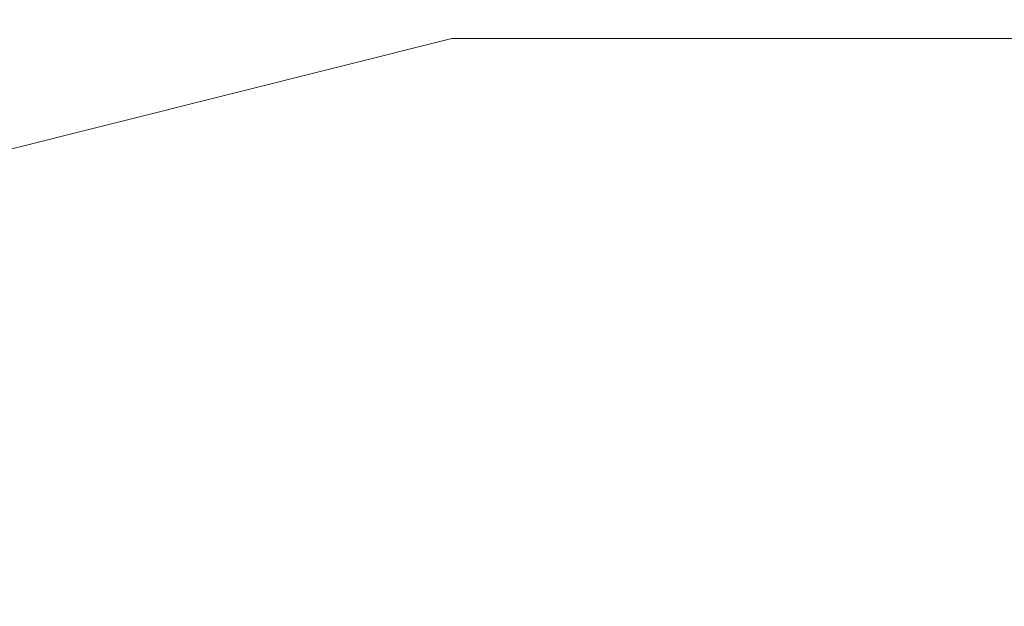
# Model space of a CAD drawing. Units: inches. Extents: x 2091 to 2899, y 967 to 2217.
# Tile 103 of 256: x 2252.951 to 2253.5204, y 1100.0709 to 1100.4099. Entities that reach past the tile are written whole.
import ezdxf

# ---------------------------------------------------------------- set-up
doc = ezdxf.new("R2010")
doc.units = ezdxf.units.IN
doc.layers.add('A-ANNO-DIMS', color=2, linetype='Continuous', lineweight=18)
doc.layers.add('L-PLNT-TREE', color=94, linetype='Continuous', lineweight=13)
doc.layers.add('A-WALL-PATT', color=141, linetype='Continuous', lineweight=13, true_color=0xadddf7)
doc.styles.get("Standard").update_dxf_attribs({"font": 'arial.ttf'})
doc.dimstyles.new('ISO-25', dxfattribs={"dimtxt": 4, "dimasz": 4, "dimexe": 1.25, "dimexo": 0.625, "dimtad": 1, "dimdec": 0, "dimlunit": 3, "dimtxsty": 'Standard', "dimcen": 2.5, "dimadec": 0, "dimazin": 0, "dimtfac": 1, "dimtdec": 0, "dimtmove": 0, "dimatfit": 3, "dimfxl": 1, "dimarcsym": 0})

# ---------------------------------------------------------------- blocks, each defined once
blk = doc.blocks.new('*U29')
for p, q in [((-402.336, 12.192), (-451.104, 0)), ((-341.376, 12.192), (-402.336, 12.192))]:
    blk.add_line(p, q)
blk = doc.blocks.new('*D71')
at = {"layer": 'A-ANNO-DIMS', "color": 0, "lineweight": -2, "transparency": 16777216}
for p, q in [((2212.1436, 1351.29406), (2212.1436, 969.4643)), ((2452.1436, 1351.29406), (2452.1436, 969.4643)), ((2216.1436, 970.7143), (2448.1436, 970.7143))]:
    blk.add_line(p, q, dxfattribs=at)
at = {"layer": 'A-ANNO-DIMS', "color": 0, "transparency": 16777216}
for points in [[(2216.1436, 971.38097), (2216.1436, 970.04764), (2212.1436, 970.7143)], [(2448.1436, 971.38097), (2448.1436, 970.04764), (2452.1436, 970.7143)]]:
    blk.add_solid(points, dxfattribs=at)
at = {"layer": 'Defpoints', "color": 0, "transparency": 16777216}
for p in [(2212.1436, 1351.91906), (2452.1436, 1351.91906), (2452.1436, 970.7143)]:
    blk.add_point(p, dxfattribs=at)
at = {"layer": 'A-ANNO-DIMS', "color": 0, "transparency": 16777216, "insert": (2332.1436, 973.38159), "char_height": 4, "attachment_point": 5}
blk.add_mtext('20\'-0"', dxfattribs=at)
blk = doc.blocks.new('*D75')
at = {"layer": 'A-ANNO-DIMS', "color": 0, "lineweight": -2, "transparency": 16777216}
for p, q in [((2212.1436, 1274.79406), (2212.1436, 969.4643)), ((2308.1436, 1274.79406), (2308.1436, 969.4643)), ((2216.1436, 970.7143), (2304.1436, 970.7143))]:
    blk.add_line(p, q, dxfattribs=at)
at = {"layer": 'A-ANNO-DIMS', "color": 0, "transparency": 16777216}
for points in [[(2216.1436, 971.38097), (2216.1436, 970.04764), (2212.1436, 970.7143)], [(2304.1436, 971.38097), (2304.1436, 970.04764), (2308.1436, 970.7143)]]:
    blk.add_solid(points, dxfattribs=at)
at = {"layer": 'Defpoints', "color": 0, "transparency": 16777216}
for p in [(2212.1436, 1275.41906), (2308.1436, 1275.41906), (2308.1436, 970.7143)]:
    blk.add_point(p, dxfattribs=at)
at = {"layer": 'A-ANNO-DIMS', "color": 0, "transparency": 16777216, "insert": (2260.1436, 973.38159), "char_height": 4, "attachment_point": 5}
blk.add_mtext('8\'-0"', dxfattribs=at)

msp = doc.modelspace()

# ---------------------------------------------------------------- hatches: boundary and pattern name
at = {"layer": 'A-WALL-PATT'}
h = msp.add_hatch(color=256, dxfattribs=at)
h.dxf.hatch_style = 1
h.paths.add_polyline_path([(2803.1436, 2050.91906), (2203.1436, 2050.91906), (2203.1436, 1090.91906), (2803.1436, 1090.91906)])
h.paths.add_polyline_path([(2635.79885, 1147.54046), (2674.52405, 1147.54046, 0.376086), (2678.52967, 1152.8802), (2678.52967, 1159.55647, 0.333335), (2674.52432, 1163.56185), (2674.52432, 1163.56185), (2674.52432, 1192.93439), (2635.80597, 1192.93439), (2597.08762, 1192.93439), (2597.08762, 1163.56185, 0.333335), (2593.08228, 1159.55647), (2593.08228, 1152.8802, 0.376086), (2597.08789, 1147.54046)], flags=0)
h.paths.add_polyline_path([(2436.01043, 1278.24078, 0.000483), (2435.95264, 1278.21503, -0.001328), (2435.93563, 1278.11169, -0.001711), (2436.11644, 1278.04076, 0.002185)], flags=0)
h.paths.add_polyline_path([(2794.1436, 1143.41906), (2794.1436, 1347.41906), (2543.37017, 1347.41906), (2543.37017, 1351.91906), (2794.1436, 1351.91906), (2794.1436, 1392.71355), (2793.9474, 1392.71355), (2793.9474, 1473.5369), (2794.1436, 1473.5369), (2794.1436, 1531.91906), (2650.1436, 1531.91906), (2650.1436, 1536.41906), (2794.1436, 1536.41906), (2794.1436, 1692.41906), (2609.37561, 1692.41906), (2609.37561, 1644.41906), (2604.87561, 1644.41906), (2604.87561, 1744.91906), (2609.37561, 1744.91906), (2609.37561, 1696.91906), (2794.1436, 1696.91906), (2794.1436, 1780.91906), (2609.6436, 1780.91906), (2493.87561, 1780.91906), (2493.87561, 1785.41906), (2609.6436, 1785.41906), (2794.1436, 1785.41906), (2794.1436, 1847.93882), (2793.95122, 1847.93882), (2793.95122, 1928.76217), (2794.1436, 1928.76217), (2794.1436, 1941.41906), (2614.1436, 1941.41906), (2614.1436, 1821.41906), (2609.6436, 1821.41906), (2609.6436, 1941.41906), (2392.1436, 1941.41906), (2392.1436, 1819.91906), (2387.6436, 1819.91906), (2387.6436, 1941.41906), (2212.1436, 1941.41906), (2212.1436, 1783.91906), (2392.1436, 1783.91906), (2392.1436, 1780.91906), (2212.1436, 1780.91906), (2212.1436, 1629.41906), (2387.6436, 1629.41906), (2387.6436, 1744.91906), (2392.1436, 1744.91906), (2392.1436, 1627.91906), (2317.1436, 1627.91906), (2317.1436, 1551.41906), (2317.1436, 1536.41906), (2459.38359, 1536.41906), (2459.38359, 1602.39648), (2463.88359, 1602.39648), (2463.88359, 1531.91906), (2456.6436, 1531.91906), (2456.6436, 1529.91906), (2452.1436, 1529.91906), (2452.1436, 1531.91906), (2312.6436, 1531.91906), (2312.6436, 1551.41906), (2306.1436, 1551.41906), (2306.1436, 1555.91906), (2308.1436, 1555.91906), (2308.1436, 1551.41906), (2312.6436, 1551.41906), (2312.6436, 1627.91906), (2212.1436, 1627.91906), (2212.1436, 1555.91906), (2270.1436, 1555.91906), (2270.1436, 1551.41906), (2212.1436, 1551.41906), (2212.1436, 1351.91906), (2272.1436, 1351.91906), (2272.1436, 1347.41906), (2212.1436, 1347.41906), (2212.1436, 1275.41906), (2308.1436, 1275.41906), (2308.1436, 1351.91906), (2452.1436, 1351.91906), (2452.1436, 1493.91906), (2456.6436, 1493.91906), (2456.6436, 1347.41906), (2312.6436, 1347.41906), (2312.6436, 1270.91906), (2212.1436, 1270.91906), (2212.1436, 1099.91906), (2281.23752, 1099.91906), (2282.87104, 1110.9138), (2282.00834, 1116.9966), (2278.55774, 1121.4204), (2268.20564, 1128.0562), (2272.08764, 1128.0562), (2273.81294, 1131.927), (2279.42034, 1134.6919), (2285.02784, 1135.2449), (2287.61584, 1137.4568), (2288.04714, 1138.0098), (2289.34114, 1140.7747), (2291.06654, 1139.6687), (2292.36054, 1135.2449), (2295.37984, 1136.9038), (2296.24254, 1135.7979), (2297.10524, 1133.033), (2300.12464, 1138.0098), (2303.14394, 1138.0098), (2304.43794, 1135.7979), (2303.14394, 1133.586), (2306.59464, 1134.6919), (2307.88874, 1133.033), (2310.90804, 1135.2449), (2313.92744, 1134.1389), (2315.62686, 1132.4271), (2308.32004, 1117.5496), (2290.20384, 1109.8079), (2288.90984, 1103.1721), (2289.27231, 1099.91906), (2434.91823, 1099.91906), (2431.59323, 1124.78806), (2429.93023, 1169.55306), (2430.92718, 1240.51969), (2435.65893, 1238.18613), (2437.13523, 1196.55406), (2438.79823, 1143.97306), (2442.67823, 1111.99806), (2446.55823, 1099.91906), (2794.1436, 1099.91906), (2794.1436, 1138.91906), (2548.03245, 1138.91906), (2548.03245, 1143.41906), (2548.03245, 1148.81906), (2546.66846, 1148.03156), (2528.68569, 1179.17862, 0.256256), (2512.03245, 1148.81906), (2512.03245, 1143.41906), (2512.03245, 1138.91906), (2507.53245, 1138.91906), (2507.53245, 1143.41906), (2507.53245, 1148.81906, 0.256256), (2490.8792, 1179.17862), (2472.89644, 1148.03156), (2471.53245, 1148.81906), (2471.53245, 1143.41906), (2467.03245, 1143.41906), (2467.03245, 1269.94579, 0.039061), (2460.90999, 1273.58006), (2467.03245, 1273.58006), (2467.03245, 1286.32536, 0.014511), (2465.21619, 1286.76191), (2467.03245, 1287.05258), (2467.03245, 1323.41906), (2471.53245, 1323.41906), (2471.53245, 1148.81906), (2489.53245, 1179.99597), (2490.89644, 1179.20847), (2490.8792, 1179.17862, -0.256256), (2507.53245, 1148.81906), (2507.53245, 1143.41906), (2512.03245, 1143.41906), (2512.03245, 1148.81906, -0.256256), (2528.68569, 1179.17862), (2528.66846, 1179.20847), (2530.03245, 1179.99597), (2548.03245, 1148.81906), (2548.03245, 1143.41906)], flags=16)
h.paths.add_polyline_path([(2607.76855, 1200.94508), (2607.76855, 1265.03063), (2597.08762, 1281.05201), (2619.78459, 1281.05201), (2627.79528, 1337.12686), (2635.79885, 1337.12686), (2643.81666, 1337.12686), (2651.82736, 1281.05201), (2674.52432, 1281.05201), (2663.8434, 1265.03063), (2663.8434, 1200.94508), (2635.80597, 1200.94508)], flags=0)
edge = h.paths.add_edge_path(flags=0)
edge.add_ellipse((13303.89622, 1272.99872), major_axis=(-10595.31304, 0), ratio=0.84230387009, start_angle=0.628237219, end_angle=0.6465541, ccw=False)
edge.add_ellipse((2711.70045, 1156.85268), major_axis=(2.21977, 0), ratio=0.8423039, start_angle=111.53524, end_angle=180.62824, ccw=False)
edge.add_ellipse((13303.15629, 1272.99872), major_axis=(-10593.02631, 0), ratio=0.84230386954, start_angle=0.528271472, end_angle=0.646554097, ccw=False)
edge.add_line((2710.7646, 1175.3333), (2710.12999, 1175.3333))
edge.add_ellipse((2710.12999, 1176.57978), major_axis=(1.47985, 0), ratio=0.8423039, start_angle=180, end_angle=270, ccw=False)
edge.add_line((2708.65014, 1176.57978), (2708.65014, 1200.78291))
edge.add_ellipse((2710.12999, 1200.78291), major_axis=(1.47985, 0), ratio=0.8423039, start_angle=90, end_angle=180, ccw=False)
edge.add_line((2710.12999, 1202.02939), (2710.46508, 1202.02939))
edge.add_ellipse((13303.15629, 1272.99872), major_axis=(-10593.02631, 0), ratio=0.84230386954, start_angle=-0.090229089, end_angle=0.383866779, ccw=False)
edge.add_ellipse((2710.12999, 1290.92703), major_axis=(-1.47985, 0), ratio=0.8423039, start_angle=0, end_angle=90, ccw=False)
edge.add_line((2708.65014, 1290.92703), (2708.65014, 1315.13017))
edge.add_ellipse((2710.12999, 1315.13017), major_axis=(-1.47985, 0), ratio=0.8423039, start_angle=-90, end_angle=0, ccw=False)
edge.add_line((2710.12999, 1316.37665), (2710.70631, 1316.37665))
edge.add_ellipse((3238.40172, 1296.28957), major_axis=(528.234, 0), ratio=0.84230387, start_angle=176.3495724, end_angle=177.8200497, ccw=False)
edge.add_ellipse((2775.06304, 1071.4507), major_axis=(313.30776, 0), ratio=0.84230387, start_angle=102.1259656, end_angle=103.780529, ccw=False)
edge.add_ellipse((2775.06304, 1078.3057), major_axis=(-305.30289, 0), ratio=0.84230387, start_angle=-79.790461, end_angle=-77.5553727, ccw=False)
edge.add_ellipse((2695.14177, 1541.97538), major_axis=(-250.96022, 0), ratio=0.84230387, start_angle=99.256566, end_angle=102.5549326)
edge.add_line((2741.41033, 1334.21426), (2747.13255, 1337.37848))
edge.add_ellipse((2747.53862, 1336.85748), major_axis=(-0.73992, 0), ratio=0.842304, start_angle=270, end_angle=307.93313, ccw=False)
edge.add_ellipse((2747.53862, 1336.85748), major_axis=(-0.73992, 0), ratio=0.842304, start_angle=232.06687, end_angle=270, ccw=False)
edge.add_line((2747.94469, 1337.37848), (2753.66691, 1334.21426))
edge.add_ellipse((2799.93547, 1541.97538), major_axis=(250.96022, 0), ratio=0.84230387, start_angle=257.4450674, end_angle=260.743434)
edge.add_ellipse((2720.01419, 1078.3057), major_axis=(305.30289, 0), ratio=0.84230387, start_angle=77.5553727, end_angle=79.790461, ccw=False)
edge.add_ellipse((2720.01419, 1071.4507), major_axis=(-313.30776, 0), ratio=0.84230387, start_angle=256.219471, end_angle=257.8740344, ccw=False)
edge.add_ellipse((2256.67551, 1296.28957), major_axis=(-528.234, 0), ratio=0.84230387, start_angle=182.1799503, end_angle=183.6504276, ccw=False)
edge.add_line((2784.37092, 1316.37665), (2784.94725, 1316.37665))
edge.add_ellipse((2784.94725, 1315.13017), major_axis=(1.47985, 0), ratio=0.8423039, start_angle=0, end_angle=90, ccw=False)
edge.add_line((2786.42709, 1315.13017), (2786.42709, 1290.92703))
edge.add_ellipse((2784.94725, 1290.92703), major_axis=(1.47985, 0), ratio=0.8423039, start_angle=270, end_angle=360, ccw=False)
edge.add_ellipse((-7808.07906, 1272.99872), major_axis=(10593.02631, 0), ratio=0.84230386954, start_angle=-0.383866779, end_angle=0.090229089, ccw=False)
edge.add_line((2784.61216, 1202.02939), (2784.94725, 1202.02939))
edge.add_ellipse((2784.94725, 1200.78291), major_axis=(1.47985, 0), ratio=0.8423039, start_angle=0, end_angle=90, ccw=False)
edge.add_line((2786.42709, 1200.78291), (2786.42709, 1176.57978))
edge.add_ellipse((2784.94725, 1176.57978), major_axis=(-1.47985, 0), ratio=0.8423039, start_angle=90, end_angle=180, ccw=False)
edge.add_line((2784.94725, 1175.3333), (2784.31264, 1175.3333))
edge.add_ellipse((-7808.07906, 1272.99872), major_axis=(10593.02631, 0), ratio=0.84230386954, start_angle=-0.618643196, end_angle=-0.528271472, ccw=False)
edge.add_ellipse((2783.37678, 1156.85268), major_axis=(-2.21977, 0), ratio=0.8423039, start_angle=179.37176, end_angle=248.46476, ccw=False)
edge.add_ellipse((-7808.81898, 1272.99872), major_axis=(-10595.31304, 0), ratio=0.84230386576, start_angle=179.353445923, end_angle=179.371762803, ccw=False)
edge.add_ellipse((2780.2973, 1153.50079), major_axis=(-5.24643, 0), ratio=0.8423039, start_angle=90, end_angle=179.35345, ccw=False)
edge.add_line((2780.2973, 1149.08171), (2714.77993, 1149.08171))
edge.add_ellipse((2714.77993, 1153.50079), major_axis=(5.24643, 0), ratio=0.8423039, start_angle=180.64655, end_angle=270, ccw=False)
edge = h.paths.add_edge_path(flags=0)
edge.add_line((2718.18737, 1151.00783), (2718.18737, 1170.47236))
edge.add_ellipse((2721.14706, 1170.47236), major_axis=(-2.95969, 0), ratio=0.8423039, start_angle=-90, end_angle=0, ccw=False)
edge.add_line((2721.14706, 1172.96532), (2773.93017, 1172.96532))
edge.add_ellipse((2773.93017, 1170.47236), major_axis=(-2.95969, 0), ratio=0.8423039, start_angle=180, end_angle=270, ccw=False)
edge.add_line((2776.88987, 1170.47236), (2776.88987, 1151.00783))
edge.add_line((2776.88987, 1151.00783), (2718.18737, 1151.00783))
edge = h.paths.add_edge_path(flags=0)
edge.add_line((2718.18737, 1180.23415), (2718.18737, 1199.05783))
edge.add_ellipse((2747.53862, 1320.39864), major_axis=(147.01792, 0), ratio=0.84230387, start_angle=256.4018653, end_angle=283.5981347)
edge.add_line((2776.88987, 1199.05783), (2776.88987, 1180.23415))
edge.add_ellipse((2747.53862, 1301.57496), major_axis=(147.01792, 0), ratio=0.84230387, start_angle=256.4018653, end_angle=283.5981347, ccw=False)
edge = h.paths.add_edge_path(flags=0)
edge.add_ellipse((13303.15629, 1272.99872), major_axis=(-10591.54646, 0), ratio=0.84230386955, start_angle=0.055594314, end_angle=0.377764194, ccw=False)
edge.add_line((2711.61686, 1262.72171), (2715.66741, 1249.4954))
edge.add_ellipse((6413.89196, 1241.69192), major_axis=(-3698.23616, 0), ratio=0.8423038695, start_angle=-0.12089737, end_angle=0.36407635)
edge.add_line((2715.76104, 1218.19245), (2711.93431, 1203.16736))
edge = h.paths.add_edge_path(flags=0)
edge.add_line((2718.18737, 1251.07457), (2716.00249, 1267.45044))
edge.add_ellipse((2742.15117, 1202.18954), major_axis=(81.77258, 0), ratio=0.84230387, start_angle=94.277421, end_angle=111.8349538, ccw=False)
edge.add_line((2737.00975, 1270.93063), (2758.06748, 1270.93063))
edge.add_ellipse((2752.92606, 1202.18954), major_axis=(81.77258, 0), ratio=0.84230387, start_angle=68.1650462, end_angle=85.722579, ccw=False)
edge.add_line((2779.07475, 1267.45044), (2776.88987, 1251.07457))
edge.add_ellipse((2750.33806, 1187.88536), major_axis=(79.57966, 0), ratio=0.84230387, start_angle=67.2080851, end_angle=85.1299304)
edge.add_line((2756.03466, 1254.74366), (2739.04258, 1254.74366))
edge.add_ellipse((2744.73917, 1187.88536), major_axis=(79.57966, 0), ratio=0.84230387, start_angle=94.8700696, end_angle=112.7919149)
edge = h.paths.add_edge_path(flags=0)
edge.add_line((2783.14293, 1203.16736), (2779.31619, 1218.19245))
edge.add_ellipse((-918.81473, 1241.69192), major_axis=(3698.23616, 0), ratio=0.8423038695, start_angle=-0.36407635, end_angle=0.12089737)
edge.add_line((2779.40983, 1249.4954), (2783.46037, 1262.72171))
edge.add_ellipse((-7808.07906, 1272.99872), major_axis=(-10591.54646, 0), ratio=0.84230386954, start_angle=179.622235806, end_angle=179.944405687, ccw=False)
edge = h.paths.add_edge_path(flags=0)
edge.add_ellipse((2734.20089, 1286.69044), major_axis=(-0.35661, 6.34008), ratio=0.6038336, start_angle=89.002014, end_angle=253.657408, ccw=False)
edge.add_line((2730.369, 1286.54181), (2730.369, 1301.35198))
edge.add_line((2730.369, 1301.35198), (2735.91331, 1305.2148))
edge.add_ellipse((2736.38492, 1304.73456), major_axis=(0.73992, 0), ratio=0.842304, start_angle=90, end_angle=134.48021, ccw=False)
edge.add_line((2736.38492, 1305.3578), (2738.03278, 1305.3578))
edge.add_line((2738.03278, 1305.3578), (2738.03278, 1307.70793))
edge.add_ellipse((2794.20164, 1307.70793), major_axis=(56.16886, 0), ratio=0.84230387, start_angle=150.56143, end_angle=180, ccw=False)
edge.add_ellipse((2700.87559, 1307.70793), major_axis=(-56.16886, 0), ratio=0.84230387, start_angle=180, end_angle=209.43857, ccw=False)
edge.add_line((2757.04445, 1307.70793), (2757.04445, 1305.3578))
edge.add_line((2757.04445, 1305.3578), (2758.69232, 1305.3578))
edge.add_ellipse((2758.69232, 1304.73456), major_axis=(-0.73992, 0), ratio=0.842304, start_angle=225.51979, end_angle=270, ccw=False)
edge.add_line((2759.16392, 1305.2148), (2764.70823, 1301.35198))
edge.add_line((2764.70823, 1301.35198), (2764.70823, 1286.54181))
edge.add_ellipse((2760.87634, 1286.69044), major_axis=(0.35661, 6.34008), ratio=0.6038336, start_angle=106.342592, end_angle=270.997986, ccw=False)
edge.add_line((2757.04445, 1285.79709), (2757.04445, 1307.70793))
edge.add_ellipse((2700.87559, 1307.70793), major_axis=(-56.16886, 0), ratio=0.84230387, start_angle=180, end_angle=209.43857)
edge.add_ellipse((2794.20164, 1307.70793), major_axis=(56.16886, 0), ratio=0.84230387, start_angle=150.56143, end_angle=180)
edge.add_line((2738.03278, 1307.70793), (2738.03278, 1285.79709))
h.paths.add_polyline_path([(2417.81227, 1104.4497), (2413.49227, 1102.5297), (2410.61227, 1103.9697), (2409.17227, 1106.3697), (2407.25227, 1107.3297), (2406.29227, 1109.7297), (2405.33227, 1114.0497), (2405.33227, 1117.8897), (2406.29227, 1120.1297), (2407.25227, 1119.8097), (2408.84832, 1118.32766), (2410.17395, 1119.42417), (2410.21127, 1120.4057), (2411.04073, 1121.41905), (2410.69927, 1119.8587), (2410.17395, 1119.42417), (2410.08845, 1117.17611), (2411.13284, 1116.20632), (2413.97227, 1119.3297), (2416.85227, 1120.7697), (2416.86972, 1120.79878), (2417.03507, 1119.40512), (2417.89621, 1118.14338), (2418.29227, 1118.3697), (2419.54445, 1120.03927), (2419.36092, 1118.38749), (2419.03211, 1119.35615), (2418.39894, 1118.51193), (2419.25227, 1114.5297), (2418.79409, 1107.19879)], flags=0)
h.paths.add_polyline_path([(2508.87017, 1347.41906), (2508.37017, 1347.41906), (2508.37017, 1351.91906), (2508.87017, 1351.91906)], flags=0)
h.paths.add_polyline_path([(2473.37017, 1347.41906), (2472.37017, 1347.41906), (2467.87017, 1347.41906), (2467.87017, 1455.41906), (2472.37017, 1455.41906), (2472.37017, 1352.41906), (2473.37017, 1352.41906)], flags=0)
h.paths.add_polyline_path([(2352.10624, 1217.4462), (2349.22624, 1218.8862), (2347.78624, 1221.2862), (2345.86624, 1222.2462), (2344.90624, 1224.6462), (2343.94624, 1228.9662), (2343.94624, 1232.8062), (2344.90624, 1235.0462), (2345.86624, 1234.7262), (2347.46229, 1233.24415), (2348.78792, 1234.34066), (2348.82524, 1235.3222), (2349.6547, 1236.33555), (2349.31324, 1234.7752), (2348.78792, 1234.34066), (2348.70242, 1232.0926), (2349.74681, 1231.12282), (2352.58624, 1234.2462), (2355.46624, 1235.6862), (2355.48369, 1235.71528), (2355.64904, 1234.32161), (2356.51018, 1233.05988), (2356.90624, 1233.2862), (2358.15842, 1234.95576), (2357.97489, 1233.30398), (2357.64608, 1234.27264), (2357.01291, 1233.42842), (2357.86624, 1229.4462), (2357.40806, 1222.11529), (2356.42624, 1219.3662)], flags=0)
h.paths.add_polyline_path([(2348.2968, 1112.22442), (2347.0138, 1112.31042), (2345.5298, 1114.12742), (2345.7318, 1115.85842), (2346.8118, 1116.98242), (2346.8118, 1114.64642), (2345.8668, 1114.21442), (2346.8798, 1114.30042)], flags=0)
h.paths.add_polyline_path([(2347.0138, 1110.92642), (2346.2718, 1110.49342), (2346.6098, 1111.18642)], flags=0)
h.paths.add_polyline_path([(2345.8668, 1118.19442), (2345.5298, 1117.32942), (2343.7078, 1118.02142), (2344.3828, 1118.62642)], flags=0)
h.paths.add_polyline_path([(2346.6768, 1109.28242), (2346.0698, 1108.07142), (2345.8668, 1110.06142)], flags=0)
h.paths.add_polyline_path([(2345.0568, 1119.75142), (2343.6398, 1119.75142), (2343.9778, 1121.13542)], flags=0)
h.paths.add_polyline_path([(2345.2598, 1116.55042), (2345.1248, 1115.85842), (2344.9218, 1115.68542), (2344.7198, 1116.37742)], flags=0)
h.paths.add_polyline_path([(2345.6648, 1112.31042), (2345.4618, 1111.53242), (2344.0448, 1111.96442), (2344.6518, 1112.57042)], flags=0)
h.paths.add_polyline_path([(2345.1918, 1113.34942), (2344.4498, 1113.86842), (2344.7198, 1114.38742)], flags=0)
h.paths.add_polyline_path([(2344.6518, 1116.80942), (2344.1798, 1115.68542), (2344.6518, 1115.33942), (2343.9098, 1114.90642), (2343.0328, 1115.94442), (2343.6398, 1116.46342)], flags=0)
h.paths.add_polyline_path([(2345.8668, 1106.68642), (2344.9898, 1105.56242), (2344.5168, 1106.60042)], flags=0)
h.paths.add_polyline_path([(2344.8548, 1110.06142), (2344.5168, 1109.28242), (2344.1128, 1109.71542)], flags=0)
h.paths.add_polyline_path([(2344.0448, 1113.52242), (2343.4378, 1113.08942), (2342.7628, 1113.95442)], flags=0)
h.paths.add_polyline_path([(2344.3148, 1111.01242), (2342.9648, 1110.32042), (2342.9648, 1111.09942)], flags=0)
h.paths.add_polyline_path([(2345.1248, 1104.69742), (2344.5848, 1103.74542), (2344.4498, 1104.26442)], flags=0)
h.paths.add_polyline_path([(2342.8298, 1121.22242), (2341.7498, 1120.53042), (2340.5358, 1121.04942), (2340.1308, 1121.82842), (2340.6708, 1122.95242), (2341.1428, 1121.82842), (2341.6148, 1122.00142)], flags=0)
h.paths.add_polyline_path([(2342.9648, 1119.75142), (2343.0328, 1118.45342), (2342.0878, 1118.02142), (2342.0198, 1119.49142)], flags=0)
h.paths.add_polyline_path([(2342.6948, 1116.89642), (2341.9528, 1116.63642), (2342.0198, 1117.32942)], flags=0)
h.paths.add_polyline_path([(2343.0328, 1112.22442), (2342.0198, 1111.79142), (2341.5478, 1112.22442), (2342.3578, 1113.34942)], flags=0)
h.paths.add_polyline_path([(2343.7748, 1104.43742), (2342.6278, 1102.88042), (2342.6948, 1104.61042), (2343.4378, 1105.12942)], flags=0)
h.paths.add_polyline_path([(2342.0198, 1115.07942), (2340.8058, 1115.51242), (2340.9408, 1116.37742)], flags=0)
h.paths.add_polyline_path([(2341.4808, 1120.09742), (2341.4808, 1119.40542), (2341.0758, 1119.57842), (2341.1428, 1120.09742)], flags=0)
h.paths.add_polyline_path([(2341.8178, 1114.47342), (2340.9408, 1113.08942), (2340.8058, 1114.56042)], flags=0)
h.paths.add_polyline_path([(2341.1428, 1118.54042), (2340.9408, 1116.98242), (2339.0508, 1117.67542), (2339.0508, 1118.62642)], flags=0)
h.paths.add_polyline_path([(2342.6948, 1101.66842), (2341.9528, 1101.84142), (2342.5598, 1102.36142)], flags=0)
h.paths.add_polyline_path([(2340.3328, 1119.66542), (2338.4438, 1119.57842), (2337.9038, 1120.35742), (2339.6578, 1120.61642)], flags=0)
h.paths.add_polyline_path([(2340.3328, 1115.33942), (2340.0628, 1113.69542), (2339.3878, 1115.33942)], flags=0)
h.paths.add_polyline_path([(2341.8178, 1103.83142), (2341.5478, 1102.88042), (2341.1428, 1103.65842)], flags=0)
h.paths.add_polyline_path([(2339.0508, 1122.86642), (2337.2958, 1121.82842), (2337.0938, 1123.12542), (2337.7688, 1123.81842)], flags=0)
h.paths.add_polyline_path([(2339.1178, 1121.74142), (2338.8478, 1121.22242), (2338.1738, 1121.04942), (2338.3758, 1121.56842)], flags=0)
h.paths.add_polyline_path([(2339.1858, 1119.31942), (2338.6458, 1118.71342), (2338.2408, 1118.10742), (2338.2408, 1118.88642)], flags=0)
h.paths.add_polyline_path([(2341.1428, 1101.92842), (2340.6028, 1101.23642), (2340.0628, 1101.84142), (2340.6028, 1102.36142)], flags=0)
h.paths.add_polyline_path([(2337.6338, 1117.76142), (2336.6208, 1118.28042), (2337.2958, 1118.97242)], flags=0)
h.paths.add_polyline_path([(2336.8238, 1119.57842), (2334.7988, 1118.97242), (2335.2038, 1120.35742), (2336.5538, 1120.87642)], flags=0)
h.paths.add_polyline_path([(2339.1178, 1100.45742), (2337.3638, 1100.54342), (2336.7558, 1101.23642)], flags=0)
h.paths.add_polyline_path([(2336.3508, 1122.43342), (2336.0138, 1121.91442), (2334.9338, 1122.43342), (2334.5288, 1123.47142), (2335.7438, 1122.77942)], flags=0)
h.paths.add_polyline_path([(2334.7318, 1120.87642), (2334.2588, 1120.35742), (2334.0568, 1120.78942), (2334.5968, 1121.30842)], flags=0)
h.paths.add_polyline_path([(2334.4618, 1122.17442), (2332.5718, 1121.30842), (2331.3568, 1122.17442), (2332.0998, 1122.86642)], flags=0)
h.paths.add_polyline_path([(2334.2588, 1118.54042), (2333.3818, 1118.45342), (2333.6518, 1119.31942)], flags=0)
h.paths.add_polyline_path([(2335.5418, 1102.27442), (2334.1918, 1102.62042), (2335.2718, 1103.31242)], flags=0)
h.paths.add_polyline_path([(2332.7068, 1119.66542), (2331.6948, 1120.44342), (2332.5048, 1120.78942)], flags=0)
h.paths.add_polyline_path([(2334.7318, 1101.14942), (2333.5168, 1101.58242), (2333.9888, 1101.75542)], flags=0)
h.paths.add_polyline_path([(2332.6398, 1116.63642), (2331.0868, 1116.29042), (2331.9648, 1118.19442)], flags=0)
h.paths.add_polyline_path([(2330.7498, 1121.56842), (2330.2768, 1120.27042), (2328.5228, 1119.31942), (2328.9948, 1121.04942)], flags=0)
h.paths.add_polyline_path([(2330.7498, 1118.62642), (2330.0078, 1117.50242), (2329.8728, 1118.02142)], flags=0)
h.paths.add_polyline_path([(2332.0998, 1102.36142), (2330.5468, 1102.01442), (2331.6948, 1102.96642)], flags=0)
h.paths.add_polyline_path([(2329.5348, 1113.60842), (2329.0628, 1112.31042), (2328.5898, 1113.34942)], flags=0)
h.paths.add_polyline_path([(2328.3878, 1117.84842), (2327.5098, 1116.55042), (2327.1728, 1117.76142)], flags=0)
h.paths.add_polyline_path([(2329.7378, 1106.51342), (2329.5348, 1105.30242), (2328.2528, 1106.08142)], flags=0)
h.paths.add_polyline_path([(2328.6578, 1114.38742), (2328.0498, 1114.12742), (2328.3198, 1114.90642)], flags=0)
h.paths.add_polyline_path([(2328.3198, 1112.22442), (2327.1058, 1112.13742), (2326.7008, 1112.65642)], flags=0)
h.paths.add_polyline_path([(2326.9028, 1115.25242), (2326.7008, 1114.12742), (2325.2158, 1113.60842), (2326.0928, 1115.33942)], flags=0)
h.paths.add_polyline_path([(2326.6328, 1108.33042), (2326.0928, 1107.37942), (2325.8908, 1108.50342), (2326.4978, 1109.10942)], flags=0)
h.paths.add_polyline_path([(2615.1436, 1531.91906), (2609.6436, 1531.91906), (2609.6436, 1620.41906), (2614.1436, 1620.41906), (2614.1436, 1536.41906), (2615.1436, 1536.41906)], flags=0)
h.paths.add_polyline_path([(2545.1436, 1563.41906), (2464.1436, 1563.41906), (2464.1436, 1632.41906), (2509.1436, 1632.41906), (2509.1436, 1627.91906), (2509.1436, 1603.91906), (2468.6436, 1603.91906), (2468.6436, 1567.91906), (2540.6436, 1567.91906), (2540.6436, 1591.91906), (2545.1436, 1591.91906)], flags=0)
h.paths.add_polyline_path([(2388.96905, 1549.98573), (2357.43418, 1549.98573), (2357.43418, 1623.36078), (2399.36278, 1623.36078), (2435.68947, 1623.36078), (2435.59255, 1602.55927), (2435.59255, 1602.39648), (2388.96905, 1602.39648)], flags=0)
h.paths.add_polyline_path([(2388.88063, 1555.80915), (2374.90443, 1555.80915), (2374.90443, 1600.57156), (2374.90443, 1615.45765), (2406.35088, 1615.45765), (2406.35088, 1618.93943), (2412.17429, 1615.45765), (2406.35088, 1611.97586), (2406.35088, 1615.45765), (2388.88063, 1615.45765)], flags=0)
h.paths.add_polyline_path([(2568.87561, 1644.41906), (2453.37561, 1644.41906), (2453.37561, 1785.41906), (2457.87561, 1785.41906), (2457.87561, 1648.91906), (2568.87561, 1648.91906)], flags=0)
h.paths.add_polyline_path([(2212.1436, 1945.91906), (2212.1436, 2041.91906), (2794.1436, 2041.91906), (2794.1436, 1945.91906)], flags=16)
h.paths.add_polyline_path([(2271.08273, 1964.31724), (2776.85297, 1964.31724), (2776.85297, 2037.16962), (2271.08273, 2037.16962)], flags=8)
h.paths.add_polyline_path([(2380.64929, 1536.82414), (2461.04081, 1536.82414), (2461.04081, 1554.65259), (2380.64929, 1554.65259)], flags=8)
h.paths.add_polyline_path([(2240.75571, 1609.72545), (2309.18583, 1609.72545), (2309.18583, 1617.6982), (2240.75571, 1617.6982)], flags=8)
h.paths.add_polyline_path([(2212.67726, 1313.5041), (2282.59152, 1313.5041), (2282.59152, 1322.74524), (2212.67726, 1322.74524)], flags=8)
h.paths.add_polyline_path([(2457.11198, 1114.77857), (2558.48158, 1114.77857), (2558.48158, 1142.21968), (2457.11198, 1142.21968)], flags=8)
h.paths.add_polyline_path([(2473.44234, 1273.01007), (2604.64123, 1273.01007), (2604.64123, 1318.34693), (2473.44234, 1318.34693)], flags=8)
h.paths.add_polyline_path([(2638.8763, 1626.97743), (2684.25037, 1627.97674), (2684.03848, 1637.59749), (2638.66442, 1636.59819)], flags=8)
h.paths.add_polyline_path([(2537.59055, 1453.79345), (2628.38955, 1453.79345), (2628.38955, 1475.34481), (2537.59055, 1475.34481)], flags=8)
h.paths.add_polyline_path([(2504.13764, 1714.6324), (2554.64719, 1714.6324), (2554.64719, 1730.23771), (2504.13764, 1730.23771)], flags=8)
h.paths.add_polyline_path([(2487.50118, 1575.65187), (2535.09712, 1575.65187), (2535.09712, 1598.37765), (2487.50118, 1598.37765)], flags=8)
h.paths.add_polyline_path([(2709.0994, 1735.71028), (2740.0166, 1735.71028), (2740.0166, 1749.93764), (2709.0994, 1749.93764)], flags=8)
h.paths.add_polyline_path([(2442.43842, 1792.17166), (2564.72884, 1792.17166), (2564.72884, 1842.00016), (2442.43842, 1842.00016)], flags=8)
h.paths.add_polyline_path([(2655.8158, 1809.64408), (2789.52014, 1806.6938), (2790.08498, 1832.29164), (2656.38064, 1835.24192)], flags=8)
h.paths.add_polyline_path([(2234.8427, 1797.72014), (2368.59285, 1794.76885), (2369.16072, 1820.50413), (2235.41056, 1823.45542)], flags=8)
h.paths.add_polyline_path([(2245.13847, 1644.00633), (2398.42773, 1640.6239), (2398.99484, 1666.32482), (2245.70557, 1669.70725)], flags=8)
h.paths.add_polyline_path([(2306.14285, 1431.16852), (2413.76831, 1428.79369), (2414.33315, 1454.39153), (2306.70768, 1456.76636)], flags=8)
h.paths.add_polyline_path([(2306.83458, 1458.23314), (2393.38048, 1456.32345), (2393.93281, 1481.35436), (2307.38691, 1483.26405)], flags=8)

# ---------------------------------------------------------------- block references
at = {"layer": 'L-PLNT-TREE', "xscale": 0.0393700787401575, "yscale": 0.0393700787401575, "zscale": 0.0393700787401575}
msp.add_blockref('*U29', (2269.04101, 1099.91906), dxfattribs=at)

# ---------------------------------------------------------------- dimensions: what is measured, and where the dimension line sits
at = {"layer": 'A-ANNO-DIMS'}
for base, p1, p2, picture, middle in [((2452.1436, 970.7143), (2212.1436, 1351.91906), (2452.1436, 1351.91906), '*D71', (2332.1436, 973.38159)), ((2308.1436, 970.7143), (2212.1436, 1275.41906), (2308.1436, 1275.41906), '*D75', (2260.1436, 973.38159))]:
    dim = msp.add_linear_dim(base=base, p1=p1, p2=p2, dimstyle='ISO-25', override={"dimdec": 1, "dimlfac": 1, "dimrnd": 0, "dimzin": 1, "dimdsep": 46, "dimlunit": 4, "dimfrac": 2}, dxfattribs=at)
    dim.commit()
    dim.dimension.update_dxf_attribs({"geometry": picture, "text_midpoint": middle})

doc.saveas('drawing.dxf')
